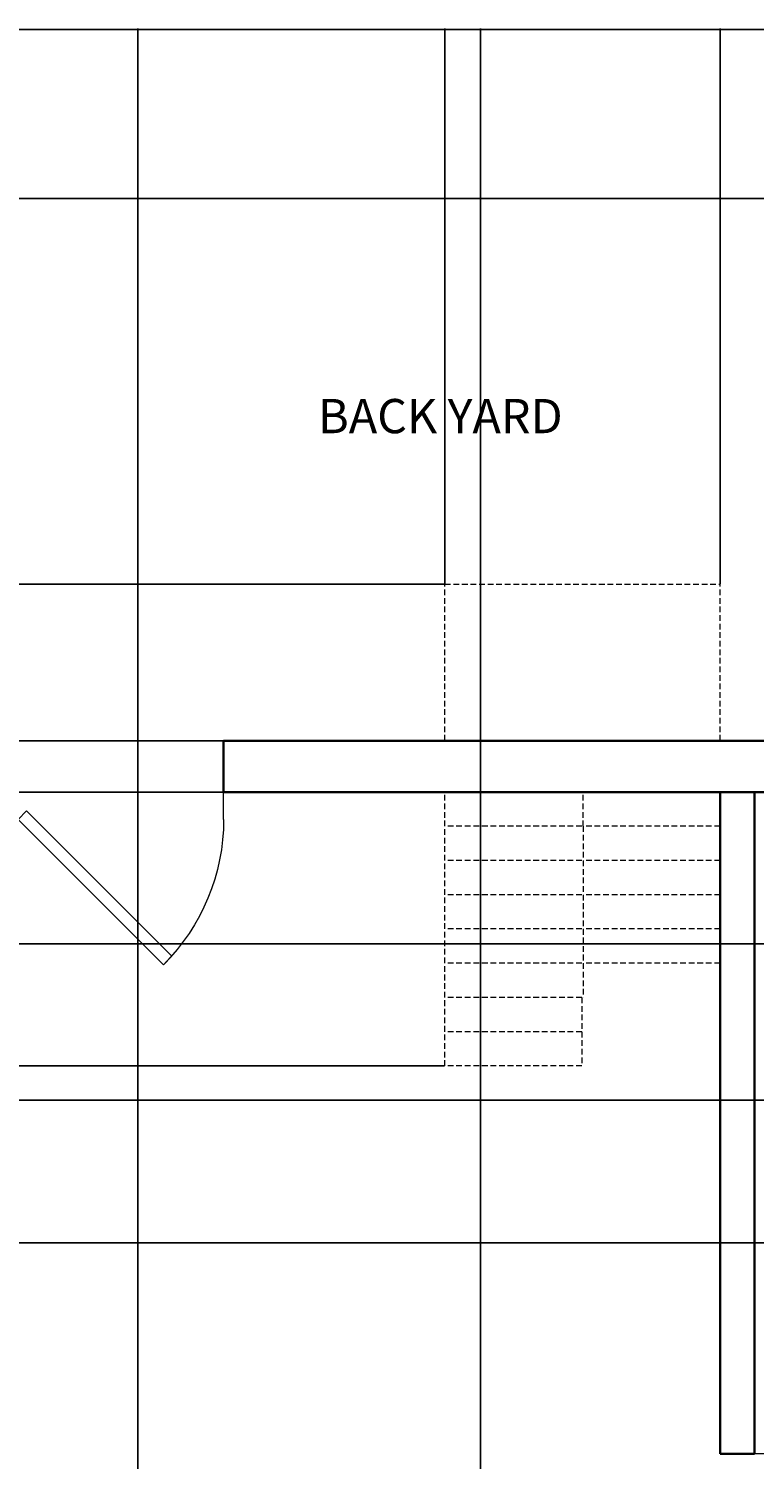
# Model space of a CAD drawing. Units: inches. Extents: x 450 to 1026, y 542 to 1190.
# Tile 10 of 11: x 698 to 826, y 939 to 1190. Entities that reach past the tile are written whole.
import ezdxf

# ---------------------------------------------------------------- set-up
doc = ezdxf.new("R2010")
doc.units = ezdxf.units.IN
doc.header["$MEASUREMENT"] = 0
doc.linetypes.add('DASHEDX2', pattern=[1.5, 1, -0.5])
for name, color, linetype, lineweight in [('A-ANNO-DIMS', 2, 'Continuous', 18), ('A-AREA-IDEN', 7, 'Continuous', 18), ('A-DOOR', 4, 'Continuous', 18), ('A-FLOR-STRS-OVHD', 8, 'DASHEDX2', 18), ('A-WALL', 7, 'Continuous', 35), ('C-PROP', 7, 'Continuous', 25)]:
    doc.layers.add(name, color=color, linetype=linetype, lineweight=lineweight)
doc.styles.get("Standard").update_dxf_attribs({"font": 'arial.ttf'})
doc.dimstyles.get("Standard").update_dxf_attribs({"dimtxt": 0.18, "dimasz": 0.18, "dimexe": 0.18, "dimexo": 0.0625, "dimgap": 0.09, "dimtad": 0, "dimtih": 1, "dimtoh": 1, "dimdec": 4, "dimzin": 0, "dimdsep": 46, "dimtxsty": 'Standard', "dimcen": 0.09, "dimadec": 0, "dimazin": 0, "dimtfac": 1, "dimtdec": 4, "dimtofl": 0, "dimtmove": 0, "dimatfit": 3, "dimfxl": 1, "dimtolj": 1, "dimtzin": 0, "dimarcsym": 0})

# ---------------------------------------------------------------- blocks, each defined once
blk = doc.blocks.new('*U4')
for p, q in [((0, 0), (0, -100)), ((750, 0), (750, -100))]:
    blk.add_line(p, q)
blk.add_lwpolyline([(0, 0), (530.3, 530.3), (561.3, 499.4), (30.9, -30.9)], close=True)
blk.add_arc((0, 0), 750, 0, 45)
blk = doc.blocks.new('*D47')
at = {"layer": 'A-ANNO-DIMS', "color": 0, "lineweight": -2, "transparency": 16777216}
for p, q in [((479.65, 1160.01), (479.65, 1189.72)), ((479.83, 1189.54), (719.36, 1189.54)), ((959.47, 1189.54), (719.94, 1189.54)), ((959.65, 1065.01), (959.65, 1189.72))]:
    blk.add_line(p, q, dxfattribs=at)
at = {"layer": 'A-ANNO-DIMS', "color": 0, "transparency": 16777216}
for points in [[(479.83, 1189.57), (479.83, 1189.51), (479.65, 1189.54)], [(959.47, 1189.57), (959.47, 1189.51), (959.65, 1189.54)]]:
    blk.add_solid(points, dxfattribs=at)
at = {"layer": 'Defpoints', "color": 0, "transparency": 16777216}
for p in [(959.65, 1189.54), (479.65, 1159.94), (959.65, 1064.94)]:
    blk.add_point(p, dxfattribs=at)
at = {"layer": 'A-ANNO-DIMS', "color": 0, "transparency": 16777216, "insert": (719.65, 1189.54), "char_height": 0.18, "attachment_point": 5}
blk.add_mtext('\\A1;480', dxfattribs=at)
blk = doc.blocks.new('*D55')
at = {"layer": 'A-ANNO-DIMS', "color": 0, "lineweight": -2, "transparency": 16777216}
for p, q in [((995.59, 1159.94), (449.87, 1159.94)), ((450.05, 1159.76), (450.05, 1112.62)), ((450.05, 1065.12), (450.05, 1112.26)), ((959.59, 1064.94), (449.87, 1064.94))]:
    blk.add_line(p, q, dxfattribs=at)
at = {"layer": 'A-ANNO-DIMS', "color": 0, "transparency": 16777216}
for points in [[(450.02, 1159.76), (450.08, 1159.76), (450.05, 1159.94)], [(450.02, 1065.12), (450.08, 1065.12), (450.05, 1064.94)]]:
    blk.add_solid(points, dxfattribs=at)
at = {"layer": 'Defpoints', "color": 0, "transparency": 16777216}
for p in [(995.65, 1159.94), (450.05, 1064.94), (959.65, 1064.94)]:
    blk.add_point(p, dxfattribs=at)
at = {"layer": 'A-ANNO-DIMS', "color": 0, "transparency": 16777216, "insert": (450.05, 1112.44), "char_height": 0.18, "attachment_point": 5}
blk.add_mtext('\\A1;95', dxfattribs=at)
blk = doc.blocks.new('*D60')
at = {"layer": 'A-ANNO-DIMS', "color": 0, "lineweight": -2, "transparency": 16777216}
for p, q in [((717.65, 827.01), (717.65, 1189.72)), ((717.83, 1189.54), (747.43, 1189.54)), ((777.47, 1189.54), (747.87, 1189.54)), ((777.65, 827.01), (777.65, 1189.72))]:
    blk.add_line(p, q, dxfattribs=at)
at = {"layer": 'A-ANNO-DIMS', "color": 0, "transparency": 16777216}
for points in [[(717.83, 1189.57), (717.83, 1189.51), (717.65, 1189.54)], [(777.47, 1189.57), (777.47, 1189.51), (777.65, 1189.54)]]:
    blk.add_solid(points, dxfattribs=at)
at = {"layer": 'Defpoints', "color": 0, "transparency": 16777216}
for p in [(777.65, 1189.54), (717.65, 826.94), (777.65, 826.94)]:
    blk.add_point(p, dxfattribs=at)
at = {"layer": 'A-ANNO-DIMS', "color": 0, "transparency": 16777216, "insert": (747.65, 1189.54), "char_height": 0.18, "attachment_point": 5}
blk.add_mtext('\\A1;60', dxfattribs=at)
blk = doc.blocks.new('*D61')
at = {"layer": 'A-ANNO-DIMS', "color": 0, "lineweight": -2, "transparency": 16777216}
for p, q in [((771.42, 1092.42), (771.42, 1189.72)), ((771.6, 1189.54), (795.14, 1189.54)), ((819.47, 1189.54), (795.93, 1189.54)), ((819.65, 1092.42), (819.65, 1189.72))]:
    blk.add_line(p, q, dxfattribs=at)
at = {"layer": 'A-ANNO-DIMS', "color": 0, "transparency": 16777216}
for points in [[(771.6, 1189.57), (771.6, 1189.51), (771.42, 1189.54)], [(819.47, 1189.57), (819.47, 1189.51), (819.65, 1189.54)]]:
    blk.add_solid(points, dxfattribs=at)
at = {"layer": 'Defpoints', "color": 0, "transparency": 16777216}
for p in [(819.65, 1189.54), (771.42, 1092.35), (819.65, 1092.35)]:
    blk.add_point(p, dxfattribs=at)
at = {"layer": 'A-ANNO-DIMS', "color": 0, "transparency": 16777216, "insert": (795.54, 1189.54), "char_height": 0.18, "attachment_point": 5}
blk.add_mtext('\\A1;48.23', dxfattribs=at)
blk = doc.blocks.new('*D62')
at = {"layer": 'A-ANNO-DIMS', "color": 0, "lineweight": -2, "transparency": 16777216}
for p, q in [((771.36, 1055.94), (449.87, 1055.94)), ((450.05, 1055.76), (450.05, 1032.12)), ((450.05, 1008.12), (450.05, 1031.76)), ((771.36, 1007.94), (449.87, 1007.94))]:
    blk.add_line(p, q, dxfattribs=at)
at = {"layer": 'A-ANNO-DIMS', "color": 0, "transparency": 16777216}
for points in [[(450.02, 1055.76), (450.08, 1055.76), (450.05, 1055.94)], [(450.02, 1008.12), (450.08, 1008.12), (450.05, 1007.94)]]:
    blk.add_solid(points, dxfattribs=at)
at = {"layer": 'Defpoints', "color": 0, "transparency": 16777216}
for p in [(771.42, 1055.94), (450.05, 1007.94), (771.42, 1007.94)]:
    blk.add_point(p, dxfattribs=at)
at = {"layer": 'A-ANNO-DIMS', "color": 0, "transparency": 16777216, "insert": (450.05, 1031.94), "char_height": 0.18, "attachment_point": 5}
blk.add_mtext('\\A1;48', dxfattribs=at)
blk = doc.blocks.new('*D63')
at = {"layer": 'A-ANNO-DIMS', "color": 0, "lineweight": -2, "transparency": 16777216}
for p, q in [((771.36, 1092.35), (449.87, 1092.35)), ((450.05, 1092.17), (450.05, 1078.83)), ((450.05, 1065.12), (450.05, 1078.47)), ((771.36, 1064.94), (449.87, 1064.94))]:
    blk.add_line(p, q, dxfattribs=at)
at = {"layer": 'A-ANNO-DIMS', "color": 0, "transparency": 16777216}
for points in [[(450.02, 1092.17), (450.08, 1092.17), (450.05, 1092.35)], [(450.02, 1065.12), (450.08, 1065.12), (450.05, 1064.94)]]:
    blk.add_solid(points, dxfattribs=at)
at = {"layer": 'Defpoints', "color": 0, "transparency": 16777216}
for p in [(771.42, 1092.35), (450.05, 1064.94), (771.42, 1064.94)]:
    blk.add_point(p, dxfattribs=at)
at = {"layer": 'A-ANNO-DIMS', "color": 0, "transparency": 16777216, "insert": (450.05, 1078.65), "char_height": 0.18, "attachment_point": 5}
blk.add_mtext('\\A1;27.41', dxfattribs=at)
blk = doc.blocks.new('*D68')
at = {"layer": 'A-ANNO-DIMS', "color": 0, "lineweight": -2, "transparency": 16777216}
for p, q in [((523.29, 1029.33), (1025.43, 1029.33)), ((1025.25, 1029.15), (1025.25, 1003.32)), ((1025.25, 977.12), (1025.25, 1002.96)), ((523.29, 976.94), (1025.43, 976.94))]:
    blk.add_line(p, q, dxfattribs=at)
at = {"layer": 'A-ANNO-DIMS', "color": 0, "transparency": 16777216}
for points in [[(1025.22, 1029.15), (1025.28, 1029.15), (1025.25, 1029.33)], [(1025.22, 977.12), (1025.28, 977.12), (1025.25, 976.94)]]:
    blk.add_solid(points, dxfattribs=at)
at = {"layer": 'Defpoints', "color": 0, "transparency": 16777216}
for p in [(523.22, 1029.33), (1025.25, 1029.33), (523.22, 976.94)]:
    blk.add_point(p, dxfattribs=at)
at = {"layer": 'A-ANNO-DIMS', "color": 0, "transparency": 16777216, "insert": (1025.25, 1003.14), "char_height": 0.18, "attachment_point": 5}
blk.add_mtext('\\A1;52.39', dxfattribs=at)
blk = doc.blocks.new('*D74')
at = {"layer": 'A-ANNO-DIMS', "color": 0, "lineweight": -2, "transparency": 16777216}
for p, q in [((959.59, 1055.94), (449.87, 1055.94)), ((450.05, 1055.76), (450.05, 1029.12)), ((450.05, 1002.12), (450.05, 1028.76)), ((950.59, 1001.94), (449.87, 1001.94))]:
    blk.add_line(p, q, dxfattribs=at)
at = {"layer": 'A-ANNO-DIMS', "color": 0, "transparency": 16777216}
for points in [[(450.02, 1055.76), (450.08, 1055.76), (450.05, 1055.94)], [(450.02, 1002.12), (450.08, 1002.12), (450.05, 1001.94)]]:
    blk.add_solid(points, dxfattribs=at)
at = {"layer": 'Defpoints', "color": 0, "transparency": 16777216}
for p in [(450.05, 1055.94), (959.65, 1055.94), (950.65, 1001.94)]:
    blk.add_point(p, dxfattribs=at)
at = {"layer": 'A-ANNO-DIMS', "color": 0, "transparency": 16777216, "insert": (450.05, 1028.94), "char_height": 0.18, "attachment_point": 5}
blk.add_mtext('\\A1;54', dxfattribs=at)

msp = doc.modelspace()

# ---------------------------------------------------------------- linework, layer by layer
at = {"layer": 'A-FLOR-STRS-OVHD'}
for p, q in [((771.4199, 1064.9426), (771.4199, 1092.353)), ((771.4199, 1092.353), (819.6513, 1092.353)), ((819.6513, 1064.9426), (819.6513, 1092.353)), ((771.4199, 1007.9426), (771.4199, 1055.9426)), ((795.6513, 1049.9426), (795.6513, 1055.9426)), ((819.6513, 1055.9426), (819.6513, 1049.9426)), ((795.4199, 1049.9426), (771.4199, 1049.9426)), ((819.6513, 1049.9426), (795.6513, 1049.9426)), ((795.6513, 1049.9426), (795.6513, 1019.9426)), ((795.4199, 1043.9426), (771.4199, 1043.9426)), ((819.6513, 1043.9426), (795.6513, 1043.9426)), ((795.4199, 1037.9426), (771.4199, 1037.9426)), ((819.6513, 1037.9426), (795.6513, 1037.9426)), ((795.4199, 1031.9426), (771.4199, 1031.9426)), ((819.6513, 1031.9426), (795.6513, 1031.9426)), ((795.4199, 1025.9426), (771.4199, 1025.9426)), ((819.6513, 1025.9426), (795.6513, 1025.9426)), ((795.4199, 1019.9426), (771.4199, 1019.9426)), ((795.4199, 1019.9426), (795.4199, 1007.9426)), ((795.4199, 1013.9426), (771.4199, 1013.9426)), ((795.4199, 1007.9426), (771.4199, 1007.9426))]:
    msp.add_line(p, q, dxfattribs=at)
at = {"layer": 'A-WALL'}
for p, q in [((732.6513, 1055.9426), (732.6513, 1064.9426)), ((732.6513, 1064.9426), (959.6513, 1064.9426)), ((732.6513, 1055.9426), (959.6513, 1055.9426)), ((819.6513, 939.9426), (819.6513, 1055.9426)), ((825.6513, 939.9426), (825.6513, 1055.9426)), ((819.6513, 939.9426), (825.6513, 939.9426))]:
    msp.add_line(p, q, dxfattribs=at)
at = {"layer": 'C-PROP'}
msp.add_line((479.6513, 1159.9426), (995.6513, 1159.9426), dxfattribs=at)

# ---------------------------------------------------------------- block references
at = {"layer": 'A-DOOR', "yscale": 0.048, "zscale": 0.048}
for p, xscale, rotation in [((696.6513, 1051.1426), -0.048, 180), ((830.4513, 939.9426), 0.048, 270)]:
    msp.add_blockref('*U4', p, dxfattribs=dict(at, xscale=xscale, rotation=rotation))

# ---------------------------------------------------------------- texts
at = {"layer": 'A-AREA-IDEN'}
msp.add_text('BACK YARD', height=6, dxfattribs=at).set_placement((749.2098, 1118.8219))

# ---------------------------------------------------------------- dimensions: what is measured, and where the dimension line sits
at = {"layer": 'A-ANNO-DIMS'}
for base, p1, p2, override, picture, middle in [((959.6513, 1189.5426), (479.6513, 1159.9426), (959.6513, 1064.9426), {"dimdec": 0, "dimlfac": 1, "dimrnd": 0, "dimzin": 0, "dimdsep": 46, "dimlunit": 2}, '*D47', (719.6513, 1189.5426)), ((777.6513, 1189.5426), (717.6513, 826.9426), (777.6513, 826.9426), {"dimdec": 0, "dimlfac": 1, "dimrnd": 0, "dimzin": 0, "dimdsep": 46, "dimlunit": 2}, '*D60', (747.6513, 1189.5426)), ((819.6513, 1189.5426), (771.4199, 1092.353), (819.6513, 1092.353), {"dimdec": 2, "dimlfac": 1, "dimrnd": 0, "dimzin": 0, "dimdsep": 46, "dimlunit": 2}, '*D61', (795.5356, 1189.5426))]:
    dim = msp.add_linear_dim(base=base, p1=p1, p2=p2, dimstyle='Standard', override=override, dxfattribs=at)
    dim.commit()
    dim.dimension.update_dxf_attribs({"geometry": picture, "text_midpoint": middle})
for base, p1, p2, override, picture, middle in [((450.0513, 1064.9426), (995.6513, 1159.9426), (959.6513, 1064.9426), {"dimdec": 0, "dimlfac": 1, "dimrnd": 0, "dimzin": 0, "dimdsep": 46, "dimlunit": 2}, '*D55', (450.0513, 1112.4426)), ((450.0513, 1064.9426), (771.4199, 1092.353), (771.4199, 1064.9426), {"dimdec": 2, "dimlfac": 1, "dimrnd": 0, "dimzin": 0, "dimdsep": 46, "dimlunit": 2}, '*D63', (450.0513, 1078.6478)), ((450.0513, 1007.9426), (771.4199, 1055.9426), (771.4199, 1007.9426), {"dimdec": 0, "dimlfac": 1, "dimrnd": 0, "dimzin": 0, "dimdsep": 46, "dimlunit": 2}, '*D62', (450.0513, 1031.9426)), ((450.0513, 1055.9426), (950.6513, 1001.9426), (959.6513, 1055.9426), {"dimdec": 0, "dimlfac": 1, "dimrnd": 0, "dimzin": 0, "dimdsep": 46, "dimlunit": 2}, '*D74', (450.0513, 1028.9426)), ((1025.2513, 1029.3314), (523.2237, 976.9426), (523.2237, 1029.3314), {"dimdec": 2, "dimlfac": 1, "dimrnd": 0, "dimzin": 0, "dimdsep": 46, "dimlunit": 2}, '*D68', (1025.2513, 1003.137))]:
    dim = msp.add_linear_dim(base=base, p1=p1, p2=p2, angle=90, dimstyle='Standard', override=override, dxfattribs=at)
    dim.commit()
    dim.dimension.update_dxf_attribs({"geometry": picture, "text_midpoint": middle})

doc.saveas('drawing.dxf')
